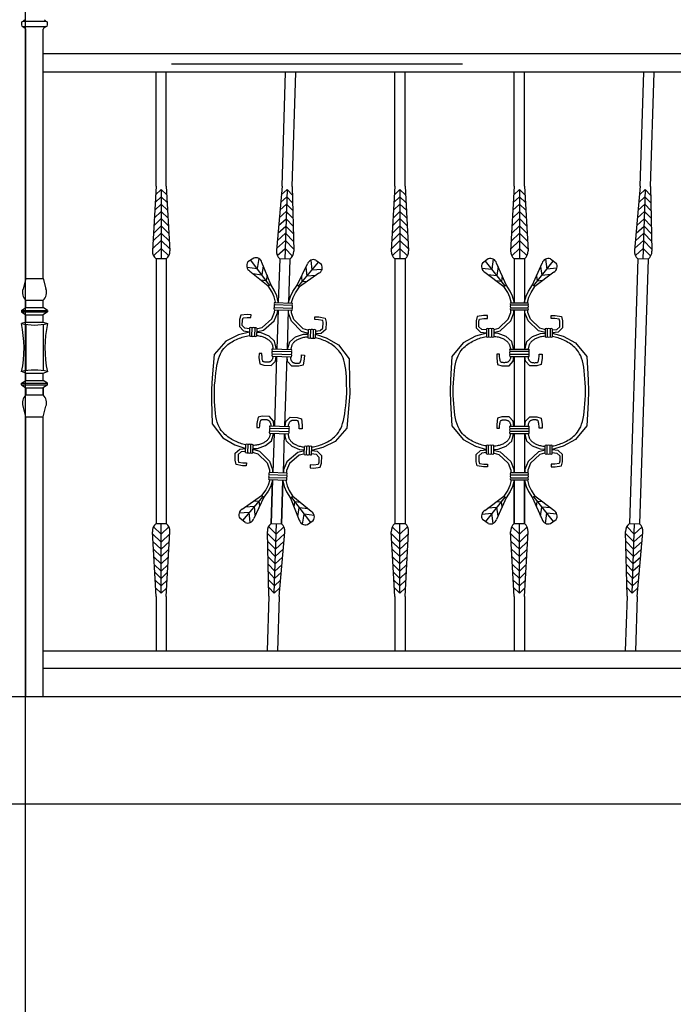
# Model space of a CAD drawing. Units: inches. Extents: x 2278 to 7495, y -71 to 1198.
# Tile 14 of 44: x 4970 to 5007, y 107 to 162. Entities that reach past the tile are written whole.
import ezdxf

# ---------------------------------------------------------------- set-up
doc = ezdxf.new("R2010")
doc.units = ezdxf.units.IN
doc.header["$MEASUREMENT"] = 0
doc.layers.add('A-ANNO-DIMS', color=2, linetype='Continuous', lineweight=18)
doc.layers.add('A-ELEV', color=7, linetype='Continuous', lineweight=25)
doc.styles.get("Standard").update_dxf_attribs({"font": 'arial.ttf'})
doc.dimstyles.get("Standard").update_dxf_attribs({"dimtxt": 6, "dimasz": 3, "dimexe": 0.18, "dimexo": 0.0625, "dimgap": 0.09, "dimtad": 0, "dimtih": 1, "dimtoh": 1, "dimdec": 0, "dimzin": 0, "dimdsep": 46, "dimlunit": 3, "dimtxsty": 'Standard', "dimblk": 'ARCHTICK', "dimcen": 0.09, "dimadec": 0, "dimazin": 0, "dimtfac": 1, "dimtdec": 0, "dimtofl": 0, "dimtmove": 0, "dimatfit": 3, "dimfxl": 1, "dimtolj": 1, "dimtzin": 0, "dimarcsym": 0})

# ---------------------------------------------------------------- blocks, each defined once
blk = doc.blocks.new('BALUSTER-ORNATE-A')
for p, q in [((3.585, 26.003), (3.585, 32.384)), ((4.155, 26.003), (4.155, 32.38)), ((3.585, 26.003), (3.383, 22.393)), ((4.155, 26.003), (4.357, 22.393)), ((3.533, 25.084), (3.87, 25.41)), ((3.558, 25.516), (3.87, 25.818)), ((3.87, 25.818), (3.87, 21.929)), ((4.182, 25.516), (3.87, 25.818)), ((4.207, 25.084), (3.87, 25.41)), ((3.509, 24.653), (3.87, 25.001)), ((4.231, 24.653), (3.87, 25.001)), ((3.485, 24.221), (3.87, 24.593)), ((4.255, 24.221), (3.87, 24.593)), ((3.437, 23.358), (3.87, 23.777)), ((3.461, 23.79), (3.87, 24.185)), ((4.279, 23.79), (3.87, 24.185)), ((4.303, 23.358), (3.87, 23.777)), ((3.413, 22.927), (3.87, 23.369)), ((4.327, 22.927), (3.87, 23.369)), ((3.388, 22.495), (3.87, 22.961)), ((4.352, 22.495), (3.87, 22.961)), ((3.442, 22.106), (3.87, 22.52)), ((4.299, 22.106), (3.87, 22.52)), ((2.128, 21.929), (1.813, 21.699)), ((3.063, 20.442), (1.97, 21.814)), ((2.412, 21.914), (2.339, 21.352)), ((3.131, 20.487), (2.594, 21.696)), ((2.678, 21.507), (2.613, 21.007)), ((3.585, 21.929), (3.585, 19.485)), ((4.155, 21.929), (3.585, 21.929)), ((4.155, 21.929), (4.155, 19.485)), ((4.609, 20.487), (5.146, 21.696)), ((4.677, 20.442), (5.77, 21.814)), ((5.062, 21.507), (5.127, 21.007)), ((5.328, 21.914), (5.401, 21.352)), ((5.612, 21.929), (5.927, 21.699)), ((1.774, 21.406), (2.339, 21.352)), ((1.936, 21.192), (2.995, 20.398)), ((2.111, 21.055), (2.613, 21.007)), ((2.907, 20.992), (2.868, 20.688)), ((5.804, 21.192), (4.745, 20.398)), ((4.833, 20.992), (4.872, 20.688)), ((5.629, 21.055), (5.127, 21.007)), ((5.966, 21.406), (5.401, 21.352)), ((2.562, 20.717), (2.868, 20.688)), ((2.995, 20.398), (3.131, 20.487)), ((3.217, 20.057), (2.995, 20.398)), ((3.36, 20.135), (3.131, 20.487)), ((4.38, 20.135), (4.609, 20.487)), ((4.523, 20.057), (4.745, 20.398)), ((4.745, 20.398), (4.609, 20.487)), ((5.178, 20.717), (4.872, 20.688)), ((3.337, 19.795), (3.217, 20.057)), ((3.49, 19.852), (3.36, 20.135)), ((3.585, 19.526), (3.49, 19.852)), ((4.155, 19.526), (4.25, 19.852)), ((4.25, 19.852), (4.38, 20.135)), ((4.403, 19.795), (4.523, 20.057)), ((3.421, 19.506), (3.337, 19.795)), ((3.37, 19.485), (4.37, 19.485)), ((3.37, 19.363), (4.37, 19.363)), ((3.42, 19.485), (3.421, 19.506)), ((3.583, 19.485), (3.585, 19.526)), ((4.157, 19.485), (4.155, 19.526)), ((4.319, 19.506), (4.403, 19.795)), ((4.32, 19.485), (4.319, 19.506)), ((1.866, 18.759), (1.513, 18.705)), ((2.084, 18.759), (1.866, 18.759)), ((2.084, 18.596), (2.084, 18.759)), ((3.247, 18.557), (3.396, 18.942)), ((3.37, 19.2), (4.37, 19.2)), ((3.37, 19.077), (4.37, 19.077)), ((3.385, 18.463), (3.558, 18.908)), ((3.396, 18.942), (3.402, 19.077)), ((3.558, 18.908), (3.565, 19.077)), ((3.585, 19.077), (3.585, 16.887)), ((4.155, 19.077), (4.155, 16.887)), ((4.182, 18.908), (4.175, 19.077)), ((4.355, 18.463), (4.182, 18.908)), ((4.344, 18.942), (4.338, 19.077)), ((4.493, 18.557), (4.344, 18.942)), ((5.656, 18.596), (5.656, 18.759)), ((5.656, 18.759), (5.874, 18.759)), ((5.874, 18.759), (6.227, 18.705)), ((1.513, 18.705), (1.449, 18.469)), ((1.449, 18.469), (1.449, 18.069)), ((1.612, 18.447), (1.642, 18.56)), ((1.612, 18.138), (1.612, 18.447)), ((1.642, 18.56), (1.879, 18.596)), ((1.879, 18.596), (2.084, 18.596)), ((2.719, 18.062), (3.247, 18.557)), ((2.801, 17.915), (3.385, 18.463)), ((4.939, 17.915), (4.355, 18.463)), ((5.021, 18.062), (4.493, 18.557)), ((5.861, 18.596), (5.656, 18.596)), ((6.098, 18.56), (5.861, 18.596)), ((6.128, 18.447), (6.098, 18.56)), ((6.128, 18.138), (6.128, 18.447)), ((6.227, 18.705), (6.291, 18.469)), ((6.291, 18.469), (6.291, 18.069)), ((2.026, 17.782), (1.412, 17.603)), ((1.449, 18.069), (1.694, 17.833)), ((1.767, 17.989), (1.612, 18.138)), ((1.694, 17.833), (2.026, 17.797)), ((2.026, 17.961), (1.767, 17.989)), ((2.026, 18.021), (2.026, 17.565)), ((2.148, 18.021), (2.148, 17.565)), ((2.311, 18.021), (2.311, 17.565)), ((2.434, 18.021), (2.434, 17.565)), ((2.434, 17.99), (2.462, 17.993)), ((2.434, 17.826), (2.492, 17.833)), ((2.683, 17.766), (2.434, 17.777)), ((2.462, 17.993), (2.719, 18.062)), ((2.492, 17.833), (2.801, 17.915)), ((3.128, 17.594), (2.683, 17.766)), ((4.612, 17.594), (5.057, 17.766)), ((5.248, 17.833), (4.939, 17.915)), ((5.278, 17.993), (5.021, 18.062)), ((5.057, 17.766), (5.306, 17.777)), ((5.306, 17.826), (5.248, 17.833)), ((5.306, 17.99), (5.278, 17.993)), ((5.306, 18.021), (5.306, 17.565)), ((5.429, 18.021), (5.429, 17.565)), ((5.592, 18.021), (5.592, 17.565)), ((5.714, 18.021), (5.714, 17.565)), ((5.714, 17.961), (5.973, 17.989)), ((6.046, 17.833), (5.714, 17.797)), ((5.714, 17.782), (6.328, 17.603)), ((5.973, 17.989), (6.128, 18.138)), ((6.291, 18.069), (6.046, 17.833)), ((0.722, 17.231), (0.096, 16.469)), ((1.412, 17.603), (0.722, 17.231)), ((0.839, 17.043), (0.916, 17.105)), ((0.916, 17.105), (0.993, 17.163)), ((0.993, 17.163), (1.071, 17.216)), ((1.071, 17.216), (1.15, 17.265)), ((1.15, 17.265), (1.23, 17.309)), ((1.23, 17.309), (1.309, 17.35)), ((1.309, 17.35), (1.389, 17.388)), ((1.389, 17.388), (1.469, 17.422)), ((1.469, 17.422), (1.549, 17.454)), ((1.549, 17.454), (1.627, 17.484)), ((1.627, 17.484), (1.705, 17.51)), ((1.705, 17.51), (1.782, 17.533)), ((1.782, 17.533), (1.858, 17.553)), ((1.858, 17.553), (1.933, 17.571)), ((1.933, 17.571), (2.007, 17.585)), ((2.007, 17.585), (2.026, 17.587)), ((2.434, 17.606), (2.499, 17.6)), ((2.499, 17.6), (2.563, 17.592)), ((2.563, 17.592), (2.624, 17.582)), ((2.624, 17.582), (2.683, 17.57)), ((2.683, 17.57), (2.739, 17.556)), ((2.739, 17.556), (2.792, 17.54)), ((2.792, 17.54), (2.843, 17.522)), ((2.843, 17.522), (2.891, 17.503)), ((2.891, 17.503), (2.937, 17.482)), ((2.937, 17.482), (2.981, 17.46)), ((2.981, 17.46), (3.024, 17.436)), ((3.024, 17.436), (3.064, 17.41)), ((3.064, 17.41), (3.102, 17.384)), ((3.102, 17.384), (3.138, 17.357)), ((3.446, 17.313), (3.128, 17.594)), ((3.138, 17.357), (3.171, 17.329)), ((3.171, 17.329), (3.201, 17.301)), ((3.201, 17.301), (3.228, 17.272)), ((3.228, 17.272), (3.252, 17.244)), ((3.252, 17.244), (3.272, 17.217)), ((3.272, 17.217), (3.288, 17.19)), ((3.288, 17.19), (3.303, 17.162)), ((3.303, 17.162), (3.316, 17.134)), ((3.316, 17.134), (3.327, 17.104)), ((3.327, 17.104), (3.337, 17.072)), ((3.528, 17.004), (3.446, 17.313)), ((4.212, 17.004), (4.294, 17.313)), ((4.294, 17.313), (4.612, 17.594)), ((4.413, 17.104), (4.403, 17.072)), ((4.424, 17.134), (4.413, 17.104)), ((4.437, 17.162), (4.424, 17.134)), ((4.452, 17.19), (4.437, 17.162)), ((4.468, 17.217), (4.452, 17.19)), ((4.489, 17.244), (4.468, 17.217)), ((4.512, 17.272), (4.489, 17.244)), ((4.539, 17.301), (4.512, 17.272)), ((4.569, 17.329), (4.539, 17.301)), ((4.602, 17.357), (4.569, 17.329)), ((4.638, 17.384), (4.602, 17.357)), ((4.676, 17.41), (4.638, 17.384)), ((4.716, 17.436), (4.676, 17.41)), ((4.759, 17.46), (4.716, 17.436)), ((4.803, 17.482), (4.759, 17.46)), ((4.849, 17.503), (4.803, 17.482)), ((4.897, 17.522), (4.849, 17.503)), ((4.948, 17.54), (4.897, 17.522)), ((5.001, 17.556), (4.948, 17.54)), ((5.057, 17.57), (5.001, 17.556)), ((5.116, 17.582), (5.057, 17.57)), ((5.177, 17.592), (5.116, 17.582)), ((5.241, 17.6), (5.177, 17.592)), ((5.306, 17.606), (5.241, 17.6)), ((5.733, 17.585), (5.714, 17.587)), ((5.807, 17.571), (5.733, 17.585)), ((5.882, 17.553), (5.807, 17.571)), ((5.958, 17.533), (5.882, 17.553)), ((6.035, 17.51), (5.958, 17.533)), ((6.113, 17.484), (6.035, 17.51)), ((6.191, 17.454), (6.113, 17.484)), ((6.271, 17.422), (6.191, 17.454)), ((6.351, 17.388), (6.271, 17.422)), ((6.328, 17.603), (7.018, 17.231)), ((6.431, 17.35), (6.351, 17.388)), ((6.51, 17.309), (6.431, 17.35)), ((6.59, 17.265), (6.51, 17.309)), ((6.669, 17.216), (6.59, 17.265)), ((6.747, 17.163), (6.669, 17.216)), ((6.824, 17.105), (6.747, 17.163)), ((6.901, 17.043), (6.824, 17.105)), ((7.018, 17.231), (7.644, 16.469)), ((0.438, 16.508), (0.495, 16.624)), ((0.495, 16.624), (0.557, 16.727)), ((0.557, 16.727), (0.623, 16.819)), ((0.623, 16.819), (0.692, 16.9)), ((0.692, 16.9), (0.764, 16.975)), ((0.764, 16.975), (0.839, 17.043)), ((2.764, 16.599), (2.602, 16.596)), ((2.602, 16.596), (2.602, 16.378)), ((2.766, 16.522), (2.764, 16.599)), ((2.769, 16.452), (2.766, 16.522)), ((3.329, 16.887), (4.411, 16.887)), ((3.329, 16.764), (4.411, 16.764)), ((3.329, 16.601), (4.411, 16.601)), ((3.337, 17.072), (3.346, 17.038)), ((3.346, 17.038), (3.354, 17.001)), ((3.354, 17.001), (3.361, 16.962)), ((3.361, 16.962), (3.368, 16.922)), ((3.368, 16.922), (3.374, 16.887)), ((3.542, 16.887), (3.528, 17.004)), ((4.198, 16.887), (4.212, 17.004)), ((4.372, 16.922), (4.366, 16.887)), ((4.379, 16.962), (4.372, 16.922)), ((4.386, 17.001), (4.379, 16.962)), ((4.394, 17.038), (4.386, 17.001)), ((4.403, 17.072), (4.394, 17.038)), ((4.971, 16.452), (4.974, 16.522)), ((4.974, 16.522), (4.976, 16.599)), ((4.976, 16.599), (5.138, 16.596)), ((5.138, 16.596), (5.138, 16.378)), ((6.976, 16.975), (6.901, 17.043)), ((7.048, 16.9), (6.976, 16.975)), ((7.117, 16.819), (7.048, 16.9)), ((7.183, 16.727), (7.117, 16.819)), ((7.245, 16.624), (7.183, 16.727)), ((7.302, 16.508), (7.245, 16.624)), ((0.096, 16.469), (0.025, 15.162)), ((0.267, 15.87), (0.3, 16.057)), ((0.3, 16.057), (0.34, 16.227)), ((0.34, 16.227), (0.386, 16.376)), ((0.386, 16.376), (0.438, 16.508)), ((2.602, 16.378), (2.656, 16.024)), ((2.656, 16.024), (2.892, 15.961)), ((2.775, 16.388), (2.769, 16.452)), ((2.783, 16.331), (2.775, 16.388)), ((2.792, 16.28), (2.783, 16.331)), ((2.803, 16.237), (2.792, 16.28)), ((2.815, 16.203), (2.803, 16.237)), ((2.825, 16.18), (2.815, 16.203)), ((2.834, 16.166), (2.825, 16.18)), ((2.84, 16.159), (2.834, 16.166)), ((2.846, 16.154), (2.84, 16.159)), ((2.852, 16.151), (2.846, 16.154)), ((2.863, 16.146), (2.852, 16.151)), ((2.88, 16.142), (2.863, 16.146)), ((2.905, 16.137), (2.88, 16.142)), ((2.936, 16.134), (2.905, 16.137)), ((2.971, 16.131), (2.936, 16.134)), ((3.008, 16.129), (2.971, 16.131)), ((3.045, 16.129), (3.008, 16.129)), ((3.081, 16.13), (3.045, 16.129)), ((3.117, 16.133), (3.081, 16.13)), ((3.15, 16.138), (3.117, 16.133)), ((3.179, 16.145), (3.15, 16.138)), ((3.205, 16.154), (3.179, 16.145)), ((3.228, 16.164), (3.205, 16.154)), ((3.249, 16.176), (3.228, 16.164)), ((3.268, 16.19), (3.249, 16.176)), ((3.286, 16.207), (3.268, 16.19)), ((3.303, 16.225), (3.286, 16.207)), ((3.292, 15.961), (3.528, 16.206)), ((3.318, 16.247), (3.303, 16.225)), ((3.333, 16.271), (3.318, 16.247)), ((3.329, 16.479), (4.411, 16.479)), ((3.346, 16.299), (3.333, 16.271)), ((3.357, 16.329), (3.346, 16.299)), ((3.368, 16.364), (3.357, 16.329)), ((3.376, 16.401), (3.368, 16.364)), ((3.383, 16.441), (3.376, 16.401)), ((3.388, 16.479), (3.383, 16.441)), ((3.528, 16.206), (3.557, 16.479)), ((3.585, 16.479), (3.585, 12.578)), ((4.155, 16.479), (4.155, 12.578)), ((4.212, 16.206), (4.183, 16.479)), ((4.448, 15.961), (4.212, 16.206)), ((4.352, 16.479), (4.357, 16.441)), ((4.357, 16.441), (4.364, 16.401)), ((4.364, 16.401), (4.372, 16.364)), ((4.372, 16.364), (4.383, 16.329)), ((4.383, 16.329), (4.394, 16.299)), ((4.394, 16.299), (4.407, 16.271)), ((4.407, 16.271), (4.422, 16.247)), ((4.422, 16.247), (4.437, 16.225)), ((4.437, 16.225), (4.454, 16.207)), ((4.454, 16.207), (4.472, 16.19)), ((4.472, 16.19), (4.491, 16.176)), ((4.491, 16.176), (4.512, 16.164)), ((4.512, 16.164), (4.535, 16.154)), ((4.535, 16.154), (4.561, 16.145)), ((4.561, 16.145), (4.59, 16.138)), ((4.59, 16.138), (4.623, 16.133)), ((4.623, 16.133), (4.659, 16.13)), ((4.659, 16.13), (4.695, 16.129)), ((4.695, 16.129), (4.732, 16.129)), ((4.732, 16.129), (4.769, 16.131)), ((4.769, 16.131), (4.804, 16.134)), ((4.804, 16.134), (4.835, 16.137)), ((4.835, 16.137), (4.86, 16.142)), ((5.084, 16.024), (4.848, 15.961)), ((4.86, 16.142), (4.877, 16.146)), ((4.877, 16.146), (4.888, 16.151)), ((4.888, 16.151), (4.895, 16.154)), ((4.895, 16.154), (4.9, 16.159)), ((4.9, 16.159), (4.906, 16.166)), ((4.906, 16.166), (4.915, 16.18)), ((4.915, 16.18), (4.925, 16.203)), ((4.925, 16.203), (4.937, 16.237)), ((4.937, 16.237), (4.948, 16.28)), ((4.948, 16.28), (4.957, 16.331)), ((4.957, 16.331), (4.965, 16.388)), ((4.965, 16.388), (4.971, 16.452)), ((5.138, 16.378), (5.084, 16.024)), ((7.354, 16.376), (7.302, 16.508)), ((7.4, 16.227), (7.354, 16.376)), ((7.44, 16.057), (7.4, 16.227)), ((7.473, 15.87), (7.44, 16.057)), ((7.644, 16.469), (7.715, 15.162)), ((0.199, 15.227), (0.217, 15.452)), ((0.217, 15.452), (0.239, 15.667)), ((0.239, 15.667), (0.267, 15.87)), ((2.892, 15.961), (3.292, 15.961)), ((4.848, 15.961), (4.448, 15.961)), ((7.501, 15.667), (7.473, 15.87)), ((7.523, 15.452), (7.501, 15.667)), ((7.541, 15.227), (7.523, 15.452)), ((0.025, 15.162), (0, 14.529)), ((0.173, 14.759), (0.185, 14.995)), ((0.185, 14.995), (0.199, 15.227)), ((7.555, 14.995), (7.541, 15.227)), ((7.567, 14.759), (7.555, 14.995)), ((7.715, 15.162), (7.74, 14.529)), ((0, 14.529), (0.025, 13.895)), ((0.163, 14.522), (0.173, 14.759)), ((0.173, 14.298), (0.163, 14.536)), ((7.577, 14.522), (7.567, 14.759)), ((7.567, 14.298), (7.577, 14.536)), ((7.74, 14.529), (7.715, 13.895)), ((0.025, 13.895), (0.096, 12.589)), ((0.185, 14.062), (0.173, 14.298)), ((0.199, 13.831), (0.185, 14.062)), ((0.217, 13.606), (0.199, 13.831)), ((7.523, 13.606), (7.541, 13.831)), ((7.541, 13.831), (7.555, 14.062)), ((7.555, 14.062), (7.567, 14.298)), ((7.715, 13.895), (7.644, 12.589)), ((0.239, 13.391), (0.217, 13.606)), ((0.267, 13.188), (0.239, 13.391)), ((7.473, 13.188), (7.501, 13.391)), ((7.501, 13.391), (7.523, 13.606)), ((0.3, 13), (0.267, 13.188)), ((0.34, 12.831), (0.3, 13)), ((0.386, 12.681), (0.34, 12.831)), ((0.438, 12.549), (0.386, 12.681)), ((2.656, 13.033), (2.602, 12.679)), ((2.602, 12.679), (2.602, 12.462)), ((2.892, 13.097), (2.656, 13.033)), ((2.769, 12.605), (2.775, 12.669)), ((2.775, 12.669), (2.783, 12.727)), ((2.783, 12.727), (2.792, 12.778)), ((2.792, 12.778), (2.803, 12.82)), ((2.803, 12.82), (2.815, 12.854)), ((2.815, 12.854), (2.825, 12.878)), ((2.825, 12.878), (2.834, 12.892)), ((2.834, 12.892), (2.84, 12.899)), ((2.84, 12.899), (2.846, 12.903)), ((2.846, 12.903), (2.852, 12.907)), ((2.852, 12.907), (2.863, 12.911)), ((2.863, 12.911), (2.88, 12.916)), ((2.88, 12.916), (2.905, 12.92)), ((3.292, 13.097), (2.892, 13.097)), ((2.905, 12.92), (2.936, 12.924)), ((2.936, 12.924), (2.971, 12.927)), ((2.971, 12.927), (3.008, 12.929)), ((3.008, 12.929), (3.045, 12.929)), ((3.045, 12.929), (3.081, 12.928)), ((3.081, 12.928), (3.117, 12.924)), ((3.117, 12.924), (3.15, 12.919)), ((3.15, 12.919), (3.179, 12.912)), ((3.179, 12.912), (3.205, 12.904)), ((3.205, 12.904), (3.228, 12.893)), ((3.228, 12.893), (3.249, 12.881)), ((3.249, 12.881), (3.268, 12.867)), ((3.268, 12.867), (3.286, 12.851)), ((3.286, 12.851), (3.303, 12.832)), ((3.528, 12.852), (3.292, 13.097)), ((3.303, 12.832), (3.318, 12.811)), ((3.318, 12.811), (3.333, 12.786)), ((3.333, 12.786), (3.346, 12.759)), ((3.346, 12.759), (3.357, 12.728)), ((3.357, 12.728), (3.368, 12.694)), ((3.368, 12.694), (3.376, 12.656)), ((3.557, 12.578), (3.528, 12.852)), ((4.183, 12.578), (4.212, 12.852)), ((4.212, 12.852), (4.448, 13.097)), ((4.372, 12.694), (4.364, 12.656)), ((4.383, 12.728), (4.372, 12.694)), ((4.394, 12.759), (4.383, 12.728)), ((4.407, 12.786), (4.394, 12.759)), ((4.422, 12.811), (4.407, 12.786)), ((4.437, 12.832), (4.422, 12.811)), ((4.454, 12.851), (4.437, 12.832)), ((4.448, 13.097), (4.848, 13.097)), ((4.472, 12.867), (4.454, 12.851)), ((4.491, 12.881), (4.472, 12.867)), ((4.512, 12.893), (4.491, 12.881)), ((4.535, 12.904), (4.512, 12.893)), ((4.561, 12.912), (4.535, 12.904)), ((4.59, 12.919), (4.561, 12.912)), ((4.623, 12.924), (4.59, 12.919)), ((4.659, 12.928), (4.623, 12.924)), ((4.695, 12.929), (4.659, 12.928)), ((4.732, 12.929), (4.695, 12.929)), ((4.769, 12.927), (4.732, 12.929)), ((4.804, 12.924), (4.769, 12.927)), ((4.835, 12.92), (4.804, 12.924)), ((4.86, 12.916), (4.835, 12.92)), ((4.848, 13.097), (5.084, 13.033)), ((4.877, 12.911), (4.86, 12.916)), ((4.888, 12.907), (4.877, 12.911)), ((4.895, 12.903), (4.888, 12.907)), ((4.9, 12.899), (4.895, 12.903)), ((4.906, 12.892), (4.9, 12.899)), ((4.915, 12.878), (4.906, 12.892)), ((4.925, 12.854), (4.915, 12.878)), ((4.937, 12.82), (4.925, 12.854)), ((4.948, 12.778), (4.937, 12.82)), ((4.957, 12.727), (4.948, 12.778)), ((4.965, 12.669), (4.957, 12.727)), ((4.971, 12.605), (4.965, 12.669)), ((5.084, 13.033), (5.138, 12.679)), ((5.138, 12.679), (5.138, 12.462)), ((7.302, 12.549), (7.354, 12.681)), ((7.354, 12.681), (7.4, 12.831)), ((7.4, 12.831), (7.44, 13)), ((7.44, 13), (7.473, 13.188)), ((0.096, 12.589), (0.722, 11.827)), ((0.495, 12.433), (0.438, 12.549)), ((0.557, 12.33), (0.495, 12.433)), ((0.623, 12.239), (0.557, 12.33)), ((0.692, 12.157), (0.623, 12.239)), ((0.764, 12.083), (0.692, 12.157)), ((2.602, 12.462), (2.764, 12.459)), ((2.764, 12.459), (2.766, 12.536)), ((2.766, 12.536), (2.769, 12.605)), ((3.329, 12.578), (4.411, 12.578)), ((3.329, 12.456), (4.411, 12.456)), ((3.329, 12.293), (4.411, 12.293)), ((3.329, 12.171), (4.411, 12.171)), ((3.368, 12.136), (3.361, 12.095)), ((3.374, 12.171), (3.368, 12.136)), ((3.376, 12.656), (3.383, 12.616)), ((3.383, 12.616), (3.388, 12.578)), ((3.528, 12.053), (3.542, 12.171)), ((3.585, 12.171), (3.585, 9.98)), ((4.155, 12.171), (4.155, 9.98)), ((4.212, 12.053), (4.198, 12.171)), ((4.357, 12.616), (4.352, 12.578)), ((4.364, 12.656), (4.357, 12.616)), ((4.366, 12.171), (4.372, 12.136)), ((4.372, 12.136), (4.379, 12.095)), ((4.974, 12.536), (4.971, 12.605)), ((4.976, 12.459), (4.974, 12.536)), ((5.138, 12.462), (4.976, 12.459)), ((6.976, 12.083), (7.048, 12.157)), ((7.644, 12.589), (7.018, 11.827)), ((7.048, 12.157), (7.117, 12.239)), ((7.117, 12.239), (7.183, 12.33)), ((7.183, 12.33), (7.245, 12.433)), ((7.245, 12.433), (7.302, 12.549)), ((0.722, 11.827), (1.412, 11.455)), ((0.839, 12.015), (0.764, 12.083)), ((0.916, 11.952), (0.839, 12.015)), ((0.993, 11.894), (0.916, 11.952)), ((1.071, 11.841), (0.993, 11.894)), ((1.15, 11.793), (1.071, 11.841)), ((1.23, 11.748), (1.15, 11.793)), ((1.309, 11.708), (1.23, 11.748)), ((1.389, 11.67), (1.309, 11.708)), ((1.469, 11.635), (1.389, 11.67)), ((1.549, 11.603), (1.469, 11.635)), ((1.627, 11.574), (1.549, 11.603)), ((1.705, 11.548), (1.627, 11.574)), ((2.937, 11.576), (2.891, 11.555)), ((2.981, 11.598), (2.937, 11.576)), ((3.024, 11.622), (2.981, 11.598)), ((3.064, 11.647), (3.024, 11.622)), ((3.102, 11.673), (3.064, 11.647)), ((3.138, 11.701), (3.102, 11.673)), ((3.128, 11.464), (3.446, 11.745)), ((3.171, 11.729), (3.138, 11.701)), ((3.201, 11.757), (3.171, 11.729)), ((3.228, 11.785), (3.201, 11.757)), ((3.252, 11.813), (3.228, 11.785)), ((3.272, 11.841), (3.252, 11.813)), ((3.288, 11.868), (3.272, 11.841)), ((3.303, 11.895), (3.288, 11.868)), ((3.316, 11.924), (3.303, 11.895)), ((3.327, 11.954), (3.316, 11.924)), ((3.337, 11.986), (3.327, 11.954)), ((3.346, 12.02), (3.337, 11.986)), ((3.354, 12.056), (3.346, 12.02)), ((3.361, 12.095), (3.354, 12.056)), ((3.446, 11.745), (3.528, 12.053)), ((4.294, 11.745), (4.212, 12.053)), ((4.612, 11.464), (4.294, 11.745)), ((4.379, 12.095), (4.386, 12.056)), ((4.386, 12.056), (4.394, 12.02)), ((4.394, 12.02), (4.403, 11.986)), ((4.403, 11.986), (4.413, 11.954)), ((4.413, 11.954), (4.424, 11.924)), ((4.424, 11.924), (4.437, 11.895)), ((4.437, 11.895), (4.452, 11.868)), ((4.452, 11.868), (4.468, 11.841)), ((4.468, 11.841), (4.489, 11.813)), ((4.489, 11.813), (4.512, 11.785)), ((4.512, 11.785), (4.539, 11.757)), ((4.539, 11.757), (4.569, 11.729)), ((4.569, 11.729), (4.602, 11.701)), ((4.602, 11.701), (4.638, 11.673)), ((4.638, 11.673), (4.676, 11.647)), ((4.676, 11.647), (4.716, 11.622)), ((4.716, 11.622), (4.759, 11.598)), ((4.759, 11.598), (4.803, 11.576)), ((4.803, 11.576), (4.849, 11.555)), ((6.035, 11.548), (6.113, 11.574)), ((6.113, 11.574), (6.191, 11.603)), ((6.191, 11.603), (6.271, 11.635)), ((6.271, 11.635), (6.351, 11.67)), ((7.018, 11.827), (6.328, 11.455)), ((6.351, 11.67), (6.431, 11.708)), ((6.431, 11.708), (6.51, 11.748)), ((6.51, 11.748), (6.59, 11.793)), ((6.59, 11.793), (6.669, 11.841)), ((6.669, 11.841), (6.747, 11.894)), ((6.747, 11.894), (6.824, 11.952)), ((6.824, 11.952), (6.901, 12.015)), ((6.901, 12.015), (6.976, 12.083)), ((1.412, 11.455), (2.026, 11.276)), ((1.449, 10.988), (1.694, 11.225)), ((1.767, 11.069), (1.612, 10.919)), ((1.694, 11.225), (2.026, 11.261)), ((1.782, 11.524), (1.705, 11.548)), ((2.026, 11.097), (1.767, 11.069)), ((1.858, 11.504), (1.782, 11.524)), ((1.933, 11.487), (1.858, 11.504)), ((2.007, 11.473), (1.933, 11.487)), ((2.026, 11.47), (2.007, 11.473)), ((2.026, 11.037), (2.026, 11.493)), ((2.148, 11.037), (2.148, 11.493)), ((2.311, 11.037), (2.311, 11.493)), ((2.434, 11.037), (2.434, 11.493)), ((2.499, 11.457), (2.434, 11.451)), ((2.434, 11.28), (2.683, 11.291)), ((2.434, 11.232), (2.492, 11.225)), ((2.434, 11.067), (2.462, 11.064)), ((2.462, 11.064), (2.719, 10.996)), ((2.492, 11.225), (2.801, 11.143)), ((2.563, 11.465), (2.499, 11.457)), ((2.624, 11.476), (2.563, 11.465)), ((2.683, 11.488), (2.624, 11.476)), ((2.739, 11.502), (2.683, 11.488)), ((2.683, 11.291), (3.128, 11.464)), ((2.792, 11.518), (2.739, 11.502)), ((2.843, 11.535), (2.792, 11.518)), ((2.801, 11.143), (3.385, 10.594)), ((2.891, 11.555), (2.843, 11.535)), ((4.939, 11.143), (4.355, 10.594)), ((5.057, 11.291), (4.612, 11.464)), ((4.849, 11.555), (4.897, 11.535)), ((4.897, 11.535), (4.948, 11.518)), ((5.248, 11.225), (4.939, 11.143)), ((4.948, 11.518), (5.001, 11.502)), ((5.001, 11.502), (5.057, 11.488)), ((5.278, 11.064), (5.021, 10.996)), ((5.057, 11.488), (5.116, 11.476)), ((5.306, 11.28), (5.057, 11.291)), ((5.116, 11.476), (5.177, 11.465)), ((5.177, 11.465), (5.241, 11.457)), ((5.241, 11.457), (5.306, 11.451)), ((5.306, 11.232), (5.248, 11.225)), ((5.306, 11.067), (5.278, 11.064)), ((5.306, 11.037), (5.306, 11.493)), ((5.429, 11.037), (5.429, 11.493)), ((5.592, 11.037), (5.592, 11.493)), ((5.714, 11.037), (5.714, 11.493)), ((5.714, 11.47), (5.733, 11.473)), ((6.328, 11.455), (5.714, 11.276)), ((6.046, 11.225), (5.714, 11.261)), ((5.714, 11.097), (5.973, 11.069)), ((5.733, 11.473), (5.807, 11.487)), ((5.807, 11.487), (5.882, 11.504)), ((5.882, 11.504), (5.958, 11.524)), ((5.958, 11.524), (6.035, 11.548)), ((5.973, 11.069), (6.128, 10.919)), ((6.291, 10.988), (6.046, 11.225)), ((1.449, 10.589), (1.449, 10.988)), ((1.513, 10.353), (1.449, 10.589)), ((1.612, 10.919), (1.612, 10.611)), ((1.612, 10.611), (1.642, 10.498)), ((1.642, 10.498), (1.879, 10.461)), ((2.719, 10.996), (3.247, 10.501)), ((3.247, 10.501), (3.396, 10.115)), ((3.385, 10.594), (3.558, 10.149)), ((4.355, 10.594), (4.182, 10.149)), ((4.493, 10.501), (4.344, 10.115)), ((5.021, 10.996), (4.493, 10.501)), ((6.098, 10.498), (5.861, 10.461)), ((6.128, 10.611), (6.098, 10.498)), ((6.128, 10.919), (6.128, 10.611)), ((6.227, 10.353), (6.291, 10.589)), ((6.291, 10.589), (6.291, 10.988)), ((1.866, 10.298), (1.513, 10.353)), ((2.084, 10.298), (1.866, 10.298)), ((1.879, 10.461), (2.084, 10.461)), ((2.084, 10.461), (2.084, 10.298)), ((3.37, 9.98), (4.37, 9.98)), ((3.396, 10.115), (3.402, 9.98)), ((3.558, 10.149), (3.565, 9.98)), ((4.182, 10.149), (4.175, 9.98)), ((4.344, 10.115), (4.338, 9.98)), ((5.861, 10.461), (5.656, 10.461)), ((5.656, 10.461), (5.656, 10.298)), ((5.656, 10.298), (5.874, 10.298)), ((5.874, 10.298), (6.227, 10.353)), ((3.421, 9.552), (3.337, 9.262)), ((3.37, 9.858), (4.37, 9.858)), ((3.37, 9.695), (4.37, 9.695)), ((3.37, 9.573), (4.37, 9.573)), ((3.42, 9.573), (3.421, 9.552)), ((3.585, 9.532), (3.49, 9.205)), ((3.583, 9.573), (3.585, 9.532)), ((3.585, 9.573), (3.585, 7.095)), ((3.585, 7.095), (3.585, 9.573)), ((4.155, 9.573), (4.155, 7.095)), ((4.155, 7.095), (4.155, 9.573)), ((4.157, 9.573), (4.155, 9.532)), ((4.155, 9.532), (4.25, 9.205)), ((4.32, 9.573), (4.319, 9.552)), ((4.319, 9.552), (4.403, 9.262)), ((3.217, 9.001), (2.995, 8.66)), ((3.36, 8.922), (3.131, 8.571)), ((3.337, 9.262), (3.217, 9.001)), ((3.49, 9.205), (3.36, 8.922)), ((4.25, 9.205), (4.38, 8.922)), ((4.38, 8.922), (4.609, 8.571)), ((4.403, 9.262), (4.523, 9.001)), ((4.523, 9.001), (4.745, 8.66)), ((1.936, 7.866), (2.995, 8.66)), ((3.063, 8.615), (1.97, 7.244)), ((2.562, 8.34), (2.868, 8.37)), ((3.131, 8.571), (2.594, 7.362)), ((2.907, 8.066), (2.868, 8.37)), ((2.995, 8.66), (3.131, 8.571)), ((4.745, 8.66), (4.609, 8.571)), ((4.609, 8.571), (5.146, 7.362)), ((4.677, 8.615), (5.77, 7.244)), ((5.804, 7.866), (4.745, 8.66)), ((4.833, 8.066), (4.872, 8.37)), ((5.178, 8.34), (4.872, 8.37)), ((2.111, 8.002), (2.613, 8.051)), ((2.678, 7.551), (2.613, 8.051)), ((5.062, 7.551), (5.127, 8.051)), ((5.629, 8.002), (5.127, 8.051)), ((1.774, 7.651), (2.339, 7.706)), ((2.128, 7.128), (1.813, 7.359)), ((2.412, 7.143), (2.339, 7.706)), ((5.328, 7.143), (5.401, 7.706)), ((5.966, 7.651), (5.401, 7.706)), ((5.612, 7.128), (5.927, 7.359)), ((3.585, 3.055), (3.383, 6.664)), ((3.442, 6.952), (3.87, 6.538)), ((3.585, 7.128), (4.155, 7.128)), ((3.87, 3.24), (3.87, 7.128)), ((4.299, 6.952), (3.87, 6.538)), ((4.155, 3.055), (4.357, 6.664)), ((3.388, 6.562), (3.87, 6.097)), ((3.413, 6.131), (3.87, 5.689)), ((4.352, 6.562), (3.87, 6.097)), ((4.327, 6.131), (3.87, 5.689)), ((3.437, 5.699), (3.87, 5.28)), ((4.303, 5.699), (3.87, 5.28)), ((3.461, 5.268), (3.87, 4.872)), ((4.279, 5.268), (3.87, 4.872)), ((3.485, 4.836), (3.87, 4.464)), ((4.255, 4.836), (3.87, 4.464)), ((3.509, 4.405), (3.87, 4.056)), ((3.533, 3.973), (3.87, 3.648)), ((4.231, 4.405), (3.87, 4.056)), ((4.207, 3.973), (3.87, 3.648)), ((3.558, 3.542), (3.87, 3.24)), ((4.182, 3.542), (3.87, 3.24)), ((3.585, 3.055), (3.585, 0)), ((4.155, 3.055), (4.155, 0))]:
    blk.add_line(p, q)
for centre, radius, start, end in [((3.929, 22.355), 0.547, 176.0178, 231.0717), ((3.811, 22.355), 0.547, 308.9283, 3.9822), ((2.111, 21.502), 0.356, 146.575, 240.6788), ((2.253, 21.595), 0.356, 16.4025, 110.5063), ((5.487, 21.595), 0.356, 69.4937, 163.5975), ((5.629, 21.502), 0.356, 299.3212, 33.425), ((3.475, 19.424), 0.121, 149.7768, 210.2232), ((3.563, 19.281), 0.209, 157.1017, 202.8983), ((4.265, 19.424), 0.121, 329.7768, 30.2232), ((4.177, 19.281), 0.209, 337.1017, 22.8983), ((3.475, 19.139), 0.121, 149.7768, 210.2232), ((4.265, 19.139), 0.121, 329.7768, 30.2232), ((2.087, 17.916), 0.121, 59.7768, 120.2232), ((2.23, 17.828), 0.209, 67.1017, 112.8983), ((2.373, 17.916), 0.121, 59.7768, 120.2232), ((5.368, 17.916), 0.121, 59.7768, 120.2232), ((5.51, 17.828), 0.209, 67.1017, 112.8983), ((5.653, 17.916), 0.121, 59.7768, 120.2232), ((2.087, 17.67), 0.121, 239.7768, 300.2232), ((2.23, 17.758), 0.209, 247.1017, 292.8983), ((2.373, 17.67), 0.121, 239.7768, 300.2232), ((5.368, 17.67), 0.121, 239.7768, 300.2232), ((5.51, 17.758), 0.209, 247.1017, 292.8983), ((5.653, 17.67), 0.121, 239.7768, 300.2232), ((3.434, 16.825), 0.121, 149.7768, 210.2232), ((3.522, 16.683), 0.209, 157.1017, 202.8983), ((3.434, 16.54), 0.121, 149.7768, 210.2232), ((4.306, 16.825), 0.121, 329.7768, 30.2232), ((4.218, 16.683), 0.209, 337.1017, 22.8983), ((4.306, 16.54), 0.121, 329.7768, 30.2232), ((3.434, 12.517), 0.121, 149.7768, 210.2232), ((3.522, 12.375), 0.209, 157.1017, 202.8983), ((3.434, 12.232), 0.121, 149.7768, 210.2232), ((4.306, 12.517), 0.121, 329.7768, 30.2232), ((4.218, 12.375), 0.209, 337.1017, 22.8983), ((4.306, 12.232), 0.121, 329.7768, 30.2232), ((2.087, 11.388), 0.121, 59.7768, 120.2232), ((2.087, 11.142), 0.121, 239.7768, 300.2232), ((2.23, 11.3), 0.209, 67.1017, 112.8983), ((2.23, 11.23), 0.209, 247.1017, 292.8983), ((2.373, 11.388), 0.121, 59.7768, 120.2232), ((2.373, 11.142), 0.121, 239.7768, 300.2232), ((5.368, 11.388), 0.121, 59.7768, 120.2232), ((5.368, 11.142), 0.121, 239.7768, 300.2232), ((5.51, 11.3), 0.209, 67.1017, 112.8983), ((5.51, 11.23), 0.209, 247.1017, 292.8983), ((5.653, 11.388), 0.121, 59.7768, 120.2232), ((5.653, 11.142), 0.121, 239.7768, 300.2232), ((3.475, 9.919), 0.121, 149.7768, 210.2232), ((4.265, 9.919), 0.121, 329.7768, 30.2232), ((3.563, 9.776), 0.209, 157.1017, 202.8983), ((3.475, 9.634), 0.121, 149.7768, 210.2232), ((4.177, 9.776), 0.209, 337.1017, 22.8983), ((4.265, 9.634), 0.121, 329.7768, 30.2232), ((2.111, 7.555), 0.356, 119.3212, 213.425), ((5.629, 7.555), 0.356, 326.575, 60.6788), ((2.253, 7.462), 0.356, 249.4937, 343.5975), ((5.487, 7.462), 0.356, 196.4025, 290.5063), ((3.929, 6.703), 0.547, 128.9283, 183.9822), ((3.811, 6.703), 0.547, 356.0178, 51.0717)]:
    blk.add_arc(centre, radius, start, end)
blk = doc.blocks.new('RAIL-BAR-A')
for p, q in [((0.202, 26.003), (0.202, 32.38)), ((0.773, 26.003), (0.773, 32.38)), ((0.202, 26.003), (0, 22.393)), ((0.773, 26.003), (0.975, 22.393)), ((0.151, 25.084), (0.488, 25.41)), ((0.175, 25.516), (0.488, 25.818)), ((0.488, 25.818), (0.488, 21.929)), ((0.8, 25.516), (0.488, 25.818)), ((0.824, 25.084), (0.488, 25.41)), ((0.127, 24.653), (0.488, 25.001)), ((0.848, 24.653), (0.488, 25.001)), ((0.103, 24.221), (0.488, 24.593)), ((0.873, 24.221), (0.488, 24.593)), ((0.054, 23.358), (0.488, 23.777)), ((0.079, 23.79), (0.488, 24.185)), ((0.897, 23.79), (0.488, 24.185)), ((0.921, 23.358), (0.488, 23.777)), ((0.03, 22.927), (0.488, 23.369)), ((0.945, 22.927), (0.488, 23.369)), ((0.006, 22.495), (0.488, 22.961)), ((0.969, 22.495), (0.488, 22.961)), ((0.059, 22.106), (0.488, 22.52)), ((0.916, 22.106), (0.488, 22.52)), ((0.202, 21.929), (0.202, 7.128)), ((0.773, 21.929), (0.202, 21.929)), ((0.773, 21.929), (0.773, 7.128)), ((0.202, 3.055), (0, 6.664)), ((0.059, 6.952), (0.488, 6.538)), ((0.202, 7.128), (0.773, 7.128)), ((0.488, 3.24), (0.488, 7.128)), ((0.916, 6.952), (0.488, 6.538)), ((0.773, 3.055), (0.975, 6.664)), ((0.006, 6.562), (0.488, 6.097)), ((0.03, 6.131), (0.488, 5.689)), ((0.969, 6.562), (0.488, 6.097)), ((0.945, 6.131), (0.488, 5.689)), ((0.054, 5.699), (0.488, 5.28)), ((0.921, 5.699), (0.488, 5.28)), ((0.079, 5.268), (0.488, 4.872)), ((0.897, 5.268), (0.488, 4.872)), ((0.103, 4.836), (0.488, 4.464)), ((0.873, 4.836), (0.488, 4.464)), ((0.127, 4.405), (0.488, 4.056)), ((0.151, 3.973), (0.488, 3.648)), ((0.848, 4.405), (0.488, 4.056)), ((0.824, 3.973), (0.488, 3.648)), ((0.175, 3.542), (0.488, 3.24)), ((0.8, 3.542), (0.488, 3.24)), ((0.202, 3.055), (0.202, 0)), ((0.773, 3.055), (0.773, 0))]:
    blk.add_line(p, q)
for centre, start, end in [((0.546, 22.355), 176.0178, 231.0717), ((0.429, 22.355), 308.9283, 3.9822), ((0.546, 6.703), 128.9283, 183.9822), ((0.429, 6.703), 356.0178, 51.0717)]:
    blk.add_arc(centre, 0.547, start, end)
blk = doc.blocks.new('RAIL-BAR-B')
for p, q in [((17.353, 32.832), (1.059, 32.832)), ((0.203, 26.003), (0.203, 32.38)), ((0.773, 26.003), (0.773, 32.38)), ((0.203, 26.003), (0.001, 22.393)), ((0.773, 26.003), (0.976, 22.393)), ((0.152, 25.084), (0.488, 25.41)), ((0.176, 25.516), (0.488, 25.818)), ((0.488, 25.818), (0.488, 21.929)), ((0.801, 25.516), (0.488, 25.818)), ((0.825, 25.084), (0.488, 25.41)), ((0.128, 24.653), (0.488, 25.001)), ((0.849, 24.653), (0.488, 25.001)), ((0.103, 24.221), (0.488, 24.593)), ((0.873, 24.221), (0.488, 24.593)), ((0.055, 23.358), (0.488, 23.777)), ((0.079, 23.79), (0.488, 24.185)), ((0.897, 23.79), (0.488, 24.185)), ((0.922, 23.358), (0.488, 23.777)), ((0.031, 22.927), (0.488, 23.369)), ((0.946, 22.927), (0.488, 23.369)), ((0.007, 22.495), (0.488, 22.961)), ((0.97, 22.495), (0.488, 22.961)), ((0.06, 22.106), (0.488, 22.52)), ((0.917, 22.106), (0.488, 22.52)), ((0.203, 21.929), (0.203, 7.128)), ((0.773, 21.929), (0.203, 21.929)), ((0.773, 21.929), (0.773, 7.128)), ((0.203, 3.055), (0.001, 6.664)), ((0.06, 6.952), (0.488, 6.538)), ((0.203, 7.128), (0.773, 7.128)), ((0.488, 3.24), (0.488, 7.128)), ((0.917, 6.952), (0.488, 6.538)), ((0.773, 3.055), (0.976, 6.664)), ((0.007, 6.562), (0.488, 6.097)), ((0.031, 6.131), (0.488, 5.689)), ((0.97, 6.562), (0.488, 6.097)), ((0.946, 6.131), (0.488, 5.689)), ((0.055, 5.699), (0.488, 5.28)), ((0.922, 5.699), (0.488, 5.28)), ((0.079, 5.268), (0.488, 4.872)), ((0.897, 5.268), (0.488, 4.872)), ((0.103, 4.836), (0.488, 4.464)), ((0.873, 4.836), (0.488, 4.464)), ((0.128, 4.405), (0.488, 4.056)), ((0.152, 3.973), (0.488, 3.648)), ((0.849, 4.405), (0.488, 4.056)), ((0.825, 3.973), (0.488, 3.648)), ((0.176, 3.542), (0.488, 3.24)), ((0.801, 3.542), (0.488, 3.24)), ((0.203, 3.055), (0.203, 0)), ((0.773, 3.055), (0.773, 0))]:
    blk.add_line(p, q)
for centre, start, end in [((0.547, 22.355), 176.0178, 231.0717), ((0.429, 22.355), 308.9283, 3.9822), ((0.547, 6.703), 128.9283, 183.9822), ((0.429, 6.703), 356.0178, 51.0717)]:
    blk.add_arc(centre, 0.547, start, end)
blk = doc.blocks.new('_ArchTick')
at = {"color": 0, "linetype": 'ByBlock', "const_width": 0.15}
blk.add_lwpolyline([(-0.5, -0.5), (0.5, 0.5)], dxfattribs=at)
blk = doc.blocks.new('*D123')
at = {"layer": 'A-ANNO-DIMS', "color": 0, "lineweight": -2, "transparency": 16777216}
for p, q in [((4736.95, 340.157), (4736.95, -23.427)), ((5145.676, -1.81), (5145.676, -23.427)), ((4736.95, -23.247), (4923.929, -23.247)), ((5145.676, -23.247), (4958.697, -23.247))]:
    blk.add_line(p, q, dxfattribs=at)
at = {"layer": 'Defpoints', "color": 0, "transparency": 16777216}
for p in [(4736.95, 340.219), (5145.676, -1.747), (5145.676, -23.247)]:
    blk.add_point(p, dxfattribs=at)
at = {"layer": 'A-ANNO-DIMS', "color": 0, "lineweight": -2, "transparency": 16777216, "xscale": 3, "yscale": 3, "zscale": 3, "rotation": 180}
blk.add_blockref('_ArchTick', (4736.95, -23.247), dxfattribs=at)
at = {"layer": 'A-ANNO-DIMS', "color": 0, "lineweight": -2, "transparency": 16777216, "xscale": 3, "yscale": 3, "zscale": 3}
blk.add_blockref('_ArchTick', (5145.676, -23.247), dxfattribs=at)
at = {"layer": 'A-ANNO-DIMS', "color": 0, "transparency": 16777216, "insert": (4941.313, -23.247), "char_height": 6, "attachment_point": 5}
blk.add_mtext('\\A1;34\'-0 1/2"', dxfattribs=at)
blk = doc.blocks.new('*D128')
at = {"layer": 'A-ANNO-DIMS', "color": 0, "lineweight": -2, "transparency": 16777216}
for p, q in [((4909.676, 99.315), (4909.676, 361.899)), ((4970.676, 60.779), (4970.676, 361.899)), ((4909.676, 361.719), (4932.111, 361.719)), ((4970.676, 361.719), (4948.241, 361.719))]:
    blk.add_line(p, q, dxfattribs=at)
at = {"layer": 'Defpoints', "color": 0, "transparency": 16777216}
for p in [(4970.676, 361.719), (4909.676, 99.253), (4970.676, 60.717)]:
    blk.add_point(p, dxfattribs=at)
at = {"layer": 'A-ANNO-DIMS', "color": 0, "lineweight": -2, "transparency": 16777216, "xscale": 3, "yscale": 3, "zscale": 3, "rotation": 180}
blk.add_blockref('_ArchTick', (4909.676, 361.719), dxfattribs=at)
at = {"layer": 'A-ANNO-DIMS', "color": 0, "lineweight": -2, "transparency": 16777216, "xscale": 3, "yscale": 3, "zscale": 3}
blk.add_blockref('_ArchTick', (4970.676, 361.719), dxfattribs=at)
at = {"layer": 'A-ANNO-DIMS', "color": 0, "transparency": 16777216, "insert": (4940.176, 361.719), "char_height": 6, "attachment_point": 5}
blk.add_mtext('\\A1;5\'-1"', dxfattribs=at)
blk = doc.blocks.new('*D129')
at = {"layer": 'A-ANNO-DIMS', "color": 0, "lineweight": -2, "transparency": 16777216}
for p, q in [((4970.676, 60.779), (4970.676, 361.899)), ((5016.176, 99.315), (5016.176, 361.899)), ((4970.676, 361.719), (4978.373, 361.719)), ((5016.176, 361.719), (5008.479, 361.719))]:
    blk.add_line(p, q, dxfattribs=at)
at = {"layer": 'Defpoints', "color": 0, "transparency": 16777216}
for p in [(5016.176, 361.719), (5016.176, 99.253), (4970.676, 60.717)]:
    blk.add_point(p, dxfattribs=at)
at = {"layer": 'A-ANNO-DIMS', "color": 0, "lineweight": -2, "transparency": 16777216, "xscale": 3, "yscale": 3, "zscale": 3, "rotation": 180}
blk.add_blockref('_ArchTick', (4970.676, 361.719), dxfattribs=at)
at = {"layer": 'A-ANNO-DIMS', "color": 0, "lineweight": -2, "transparency": 16777216, "xscale": 3, "yscale": 3, "zscale": 3}
blk.add_blockref('_ArchTick', (5016.176, 361.719), dxfattribs=at)
at = {"layer": 'A-ANNO-DIMS', "color": 0, "transparency": 16777216, "insert": (4993.426, 361.719), "char_height": 6, "attachment_point": 5}
blk.add_mtext('\\A1;3\'-9 1/2"', dxfattribs=at)

msp = doc.modelspace()

# ---------------------------------------------------------------- linework, layer by layer
at = {"layer": 'A-ELEV'}
for p, q in [((4970.676, 160.253), (4970.676, 244.253)), ((4970.451, 161.934), (4970.451, 161.816)), ((4970.533, 162.015), (4970.619, 162.112)), ((4971.836, 162.015), (4970.533, 162.015)), ((4971.836, 162.015), (4971.75, 162.112)), ((4971.918, 161.816), (4971.918, 161.934)), ((4970.533, 161.735), (4970.666, 161.64)), ((4970.533, 161.735), (4971.836, 161.735)), ((4970.696, 147.642), (4970.696, 161.577)), ((4971.673, 147.642), (4971.673, 161.577)), ((4971.836, 161.735), (4971.703, 161.64)), ((5065.039, 160.198), (4971.673, 160.198)), ((5065.039, 159.179), (4971.673, 159.179)), ((4970.696, 147.642), (4970.543, 147.049)), ((4970.696, 147.642), (4971.673, 147.642)), ((4971.673, 147.642), (4971.826, 147.049)), ((4970.451, 145.849), (4970.696, 146.012)), ((4970.696, 146.42), (4971.673, 146.42)), ((4970.696, 146.012), (4970.696, 146.42)), ((4970.696, 146.012), (4971.673, 146.012)), ((4971.673, 146.012), (4971.673, 146.42)), ((4971.918, 145.849), (4971.673, 146.012)), ((4970.451, 145.849), (4971.918, 145.849)), ((4970.451, 145.849), (4970.451, 145.768)), ((4970.451, 145.768), (4971.918, 145.768)), ((4970.451, 145.768), (4970.696, 145.605)), ((4970.696, 145.198), (4970.696, 145.605)), ((4970.696, 145.605), (4971.673, 145.605)), ((4971.918, 145.768), (4971.673, 145.605)), ((4971.673, 145.198), (4971.673, 145.605)), ((4971.918, 145.849), (4971.918, 145.768)), ((4970.696, 145.198), (4970.451, 145.116)), ((4970.696, 145.198), (4971.673, 145.198)), ((4970.696, 145.07), (4970.696, 142.474)), ((4971.673, 145.198), (4971.918, 145.116)), ((4971.673, 145.07), (4971.673, 142.474)), ((4970.696, 142.346), (4970.451, 142.428)), ((4970.696, 142.346), (4971.673, 142.346)), ((4970.696, 141.936), (4970.696, 142.346)), ((4971.673, 142.346), (4971.918, 142.428)), ((4971.673, 141.936), (4971.673, 142.346)), ((4970.451, 141.773), (4970.696, 141.936)), ((4970.451, 141.773), (4971.918, 141.773)), ((4970.451, 141.691), (4970.451, 141.773)), ((4970.451, 141.691), (4971.918, 141.691)), ((4970.451, 141.691), (4970.696, 141.529)), ((4970.696, 141.936), (4971.673, 141.936)), ((4971.918, 141.773), (4971.673, 141.936)), ((4971.918, 141.691), (4971.673, 141.529)), ((4971.918, 141.691), (4971.918, 141.773)), ((4970.696, 141.529), (4971.673, 141.529)), ((4970.696, 141.121), (4970.696, 141.529)), ((4970.696, 141.529), (4970.696, 141.121)), ((4970.696, 141.121), (4971.673, 141.121)), ((4971.673, 141.121), (4971.673, 141.529)), ((4971.673, 141.529), (4971.673, 141.121)), ((4970.696, 139.899), (4970.543, 140.492)), ((4971.673, 139.899), (4971.826, 140.492)), ((4970.696, 124.253), (4970.696, 139.899)), ((4970.696, 139.899), (4971.673, 139.899)), ((4971.673, 124.253), (4971.673, 139.899)), ((5065.039, 126.799), (4971.673, 126.799)), ((5065.039, 125.821), (4971.673, 125.821)), ((4874.676, 124.253), (5145.676, 124.253)), ((4970.676, 67.611), (4970.676, 124.253)), ((4874.676, 118.253), (5145.676, 118.253))]:
    msp.add_line(p, q, dxfattribs=at)
for centre, radius, start, end in [((4970.533, 161.934), 0.0815, 90, 180), ((4971.836, 161.934), 0.0815, 0, 90), ((4970.533, 161.816), 0.0815, 180, 270), ((4970.614, 161.577), 0.0815, 0, 50.672), ((4971.755, 161.577), 0.0815, 129.328, 180), ((4971.836, 161.816), 0.0815, 270, 360), ((4971.119, 146.856), 0.608, 161.4732, 225.8681), ((4971.25, 146.856), 0.608, 314.1319, 18.5268), ((4964.081, 143.743), 6.517, 348.3176, 12.1601), ((4971.185, 148.339), 3.305, 257.1818, 282.8182), ((4978.288, 143.743), 6.517, 167.8399, 191.6824), ((4971.185, 139.205), 3.305, 77.1818, 102.8182), ((4971.119, 140.685), 0.608, 134.1319, 198.5268), ((4971.25, 140.685), 0.608, 341.4732, 45.8681)]:
    msp.add_arc(centre, radius, start, end, dxfattribs=at)

# ---------------------------------------------------------------- block references
for name, p in [('RAIL-BAR-B', (4977.784, 126.799)), ('RAIL-BAR-A', (4991.146, 126.799)), ('BALUSTER-ORNATE-A', (4994.444, 126.799))]:
    msp.add_blockref(name, p, dxfattribs=at)
for name, p, rotation in [('BALUSTER-ORNATE-A', (4980.622, 126.93), 358.1710804743124), ('RAIL-BAR-A', (5004.04, 126.822), 358.1636620686311)]:
    msp.add_blockref(name, p, dxfattribs=dict(at, rotation=rotation))

# ---------------------------------------------------------------- dimensions: what is measured, and where the dimension line sits
at = {"layer": 'A-ANNO-DIMS'}
for base, p1, p2, picture, middle in [((5016.176, 361.719), (4970.676, 60.717), (5016.176, 99.253), '*D129', (4993.426, 361.719)), ((4970.676, 361.719), (4909.676, 99.253), (4970.676, 60.717), '*D128', (4940.176, 361.719)), ((5145.676, -23.247), (4736.95, 340.219), (5145.676, -1.747), '*D123', (4941.313, -23.247))]:
    dim = msp.add_linear_dim(base=base, p1=p1, p2=p2, dimstyle='Standard', override={"dimdec": 1, "dimlfac": 1, "dimrnd": 0, "dimzin": 1, "dimdsep": 46, "dimlunit": 4, "dimfrac": 2}, dxfattribs=at)
    dim.commit()
    dim.dimension.update_dxf_attribs({"geometry": picture, "text_midpoint": middle})

doc.saveas('drawing.dxf')
